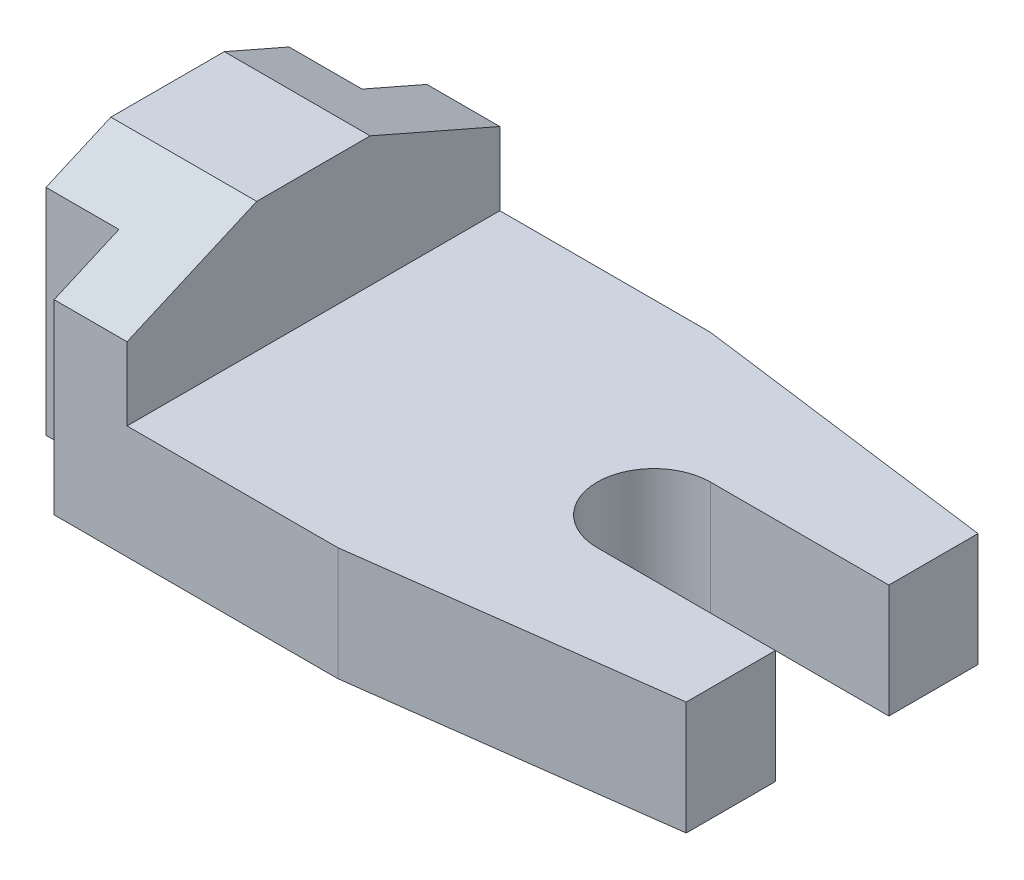
ISO-10303-21;
HEADER;
FILE_DESCRIPTION(('STEP AP214'),'2;1');
FILE_NAME('part.step','',(''),(''),'','','');
FILE_SCHEMA(('AUTOMOTIVE_DESIGN { 1 0 10303 214 1 1 1 1 }'));
ENDSEC;
DATA;
#1=APPLICATION_CONTEXT('core data for automotive mechanical design processes');
#2=APPLICATION_PROTOCOL_DEFINITION('international standard','automotive_design',2000,#1);
#3=PRODUCT_CONTEXT('',#1,'mechanical');
#4=PRODUCT('Part','Part','',(#3));
#5=PRODUCT_RELATED_PRODUCT_CATEGORY('part','',(#4));
#6=PRODUCT_DEFINITION_FORMATION('','',#4);
#7=PRODUCT_DEFINITION_CONTEXT('part definition',#1,'design');
#8=PRODUCT_DEFINITION('design','',#6,#7);
#9=PRODUCT_DEFINITION_SHAPE('','',#8);
#10=(LENGTH_UNIT() NAMED_UNIT(*) SI_UNIT(.MILLI.,.METRE.));
#11=(NAMED_UNIT(*) PLANE_ANGLE_UNIT() SI_UNIT($,.RADIAN.));
#12=(NAMED_UNIT(*) SI_UNIT($,.STERADIAN.) SOLID_ANGLE_UNIT());
#13=UNCERTAINTY_MEASURE_WITH_UNIT(LENGTH_MEASURE(1.E-05),#10,'distance_accuracy_value','');
#14=(GEOMETRIC_REPRESENTATION_CONTEXT(3) GLOBAL_UNCERTAINTY_ASSIGNED_CONTEXT((#13)) GLOBAL_UNIT_ASSIGNED_CONTEXT((#10,
#11,#12)) REPRESENTATION_CONTEXT('',''));
#15=CARTESIAN_POINT('',(0.,0.,0.));
#16=DIRECTION('',(0.,0.,1.));
#17=DIRECTION('',(1.,0.,0.));
#18=AXIS2_PLACEMENT_3D('',#15,#16,#17);
#19=CARTESIAN_POINT('',(0.,14.,0.));
#20=DIRECTION('',(0.,1.,0.));
#21=DIRECTION('',(0.,0.,1.));
#22=AXIS2_PLACEMENT_3D('',#19,#20,#21);
#23=PLANE('',#22);
#24=DIRECTION('',(1.,0.,0.));
#25=VECTOR('',#24,1.);
#26=CARTESIAN_POINT('',(0.,14.,-23.));
#27=LINE('',#26,#25);
#28=CARTESIAN_POINT('',(-4.,14.,-23.));
#29=VERTEX_POINT('',#28);
#30=CARTESIAN_POINT('',(22.,14.,-23.));
#31=VERTEX_POINT('',#30);
#32=EDGE_CURVE('E63',#29,#31,#27,.T.);
#33=ORIENTED_EDGE('',*,*,#32,.F.);
#34=DIRECTION('',(0.,0.,1.));
#35=VECTOR('',#34,1.);
#36=CARTESIAN_POINT('',(-4.,14.,0.));
#37=LINE('',#36,#35);
#38=CARTESIAN_POINT('',(-4.,14.,23.));
#39=VERTEX_POINT('',#38);
#40=EDGE_CURVE('E276',#29,#39,#37,.T.);
#41=ORIENTED_EDGE('',*,*,#40,.T.);
#42=DIRECTION('',(1.,0.,0.));
#43=VECTOR('',#42,1.);
#44=CARTESIAN_POINT('',(0.,14.,23.));
#45=LINE('',#44,#43);
#46=CARTESIAN_POINT('',(22.,14.,23.));
#47=VERTEX_POINT('',#46);
#48=EDGE_CURVE('E128',#39,#47,#45,.T.);
#49=ORIENTED_EDGE('',*,*,#48,.T.);
#50=DIRECTION('',(-0.991454295542544,0.,0.130454512571387));
#51=VECTOR('',#50,1.);
#52=CARTESIAN_POINT('',(3.34921715452689,14.,25.4540503744043));
#53=LINE('',#52,#51);
#54=CARTESIAN_POINT('',(60.,14.,18.));
#55=VERTEX_POINT('',#54);
#56=EDGE_CURVE('E253',#55,#47,#53,.T.);
#57=ORIENTED_EDGE('',*,*,#56,.F.);
#58=DIRECTION('',(0.,0.,1.));
#59=VECTOR('',#58,1.);
#60=CARTESIAN_POINT('',(60.,14.,0.));
#61=LINE('',#60,#59);
#62=CARTESIAN_POINT('',(60.,14.,7.));
#63=VERTEX_POINT('',#62);
#64=EDGE_CURVE('E257',#63,#55,#61,.T.);
#65=ORIENTED_EDGE('',*,*,#64,.F.);
#66=DIRECTION('',(-1.,0.,0.));
#67=VECTOR('',#66,1.);
#68=CARTESIAN_POINT('',(0.,14.,7.));
#69=LINE('',#68,#67);
#70=CARTESIAN_POINT('',(38.,14.,7.));
#71=VERTEX_POINT('',#70);
#72=EDGE_CURVE('E268',#63,#71,#69,.T.);
#73=ORIENTED_EDGE('',*,*,#72,.T.);
#74=CARTESIAN_POINT('',(38.,14.,0.));
#75=DIRECTION('',(0.,1.,0.));
#76=DIRECTION('',(0.,0.,1.));
#77=AXIS2_PLACEMENT_3D('',#74,#75,#76);
#78=CIRCLE('',#77,7.);
#79=CARTESIAN_POINT('',(38.,14.,-7.));
#80=VERTEX_POINT('',#79);
#81=EDGE_CURVE('E152',#80,#71,#78,.T.);
#82=ORIENTED_EDGE('',*,*,#81,.F.);
#83=DIRECTION('',(1.,0.,0.));
#84=VECTOR('',#83,1.);
#85=CARTESIAN_POINT('',(0.,14.,-7.));
#86=LINE('',#85,#84);
#87=CARTESIAN_POINT('',(60.,14.,-7.));
#88=VERTEX_POINT('',#87);
#89=EDGE_CURVE('E149',#80,#88,#86,.T.);
#90=ORIENTED_EDGE('',*,*,#89,.T.);
#91=DIRECTION('',(0.,0.,1.));
#92=VECTOR('',#91,1.);
#93=CARTESIAN_POINT('',(60.,14.,0.));
#94=LINE('',#93,#92);
#95=CARTESIAN_POINT('',(60.,14.,-18.));
#96=VERTEX_POINT('',#95);
#97=EDGE_CURVE('E155',#96,#88,#94,.T.);
#98=ORIENTED_EDGE('',*,*,#97,.F.);
#99=DIRECTION('',(-0.991454295542544,0.,-0.130454512571387));
#100=VECTOR('',#99,1.);
#101=CARTESIAN_POINT('',(3.34921715452689,14.,-25.4540503744044));
#102=LINE('',#101,#100);
#103=EDGE_CURVE('E168',#96,#31,#102,.T.);
#104=ORIENTED_EDGE('',*,*,#103,.T.);
#105=EDGE_LOOP('',(#33,#41,#49,#57,#65,#73,#82,#90,#98,#104));
#106=FACE_BOUND('',#105,.T.);
#107=ADVANCED_FACE('F50',(#106),#23,.T.);
#108=CARTESIAN_POINT('',(0.,14.,15.));
#109=DIRECTION('',(0.,0.,-1.));
#110=DIRECTION('',(-1.,0.,0.));
#111=AXIS2_PLACEMENT_3D('',#108,#109,#110);
#112=PLANE('',#111);
#113=DIRECTION('',(1.,0.,0.));
#114=VECTOR('',#113,1.);
#115=CARTESIAN_POINT('',(0.,0.,15.));
#116=LINE('',#115,#114);
#117=CARTESIAN_POINT('',(-22.,0.,15.));
#118=VERTEX_POINT('',#117);
#119=CARTESIAN_POINT('',(-13.,0.,15.));
#120=VERTEX_POINT('',#119);
#121=EDGE_CURVE('E176',#118,#120,#116,.T.);
#122=ORIENTED_EDGE('',*,*,#121,.T.);
#123=DIRECTION('',(0.,-1.,0.));
#124=VECTOR('',#123,1.);
#125=CARTESIAN_POINT('',(-13.,14.,15.));
#126=LINE('',#125,#124);
#127=CARTESIAN_POINT('',(-13.,26.5,15.));
#128=VERTEX_POINT('',#127);
#129=EDGE_CURVE('E11',#128,#120,#126,.T.);
#130=ORIENTED_EDGE('',*,*,#129,.F.);
#131=DIRECTION('',(-1.,0.,0.));
#132=VECTOR('',#131,1.);
#133=CARTESIAN_POINT('',(-13.,26.5,15.));
#134=LINE('',#133,#132);
#135=CARTESIAN_POINT('',(-22.,26.5,15.));
#136=VERTEX_POINT('',#135);
#137=EDGE_CURVE('E177',#128,#136,#134,.T.);
#138=ORIENTED_EDGE('',*,*,#137,.T.);
#139=DIRECTION('',(0.,-1.,0.));
#140=VECTOR('',#139,1.);
#141=CARTESIAN_POINT('',(-22.,14.,15.));
#142=LINE('',#141,#140);
#143=EDGE_CURVE('E121',#136,#118,#142,.T.);
#144=ORIENTED_EDGE('',*,*,#143,.T.);
#145=EDGE_LOOP('',(#122,#130,#138,#144));
#146=FACE_BOUND('',#145,.T.);
#147=ADVANCED_FACE('F47',(#146),#112,.F.);
#148=CARTESIAN_POINT('',(-13.,14.,0.));
#149=DIRECTION('',(1.,0.,0.));
#150=DIRECTION('',(0.,0.,-1.));
#151=AXIS2_PLACEMENT_3D('',#148,#149,#150);
#152=PLANE('',#151);
#153=DIRECTION('',(0.,0.,1.));
#154=VECTOR('',#153,1.);
#155=CARTESIAN_POINT('',(-13.,0.,0.));
#156=LINE('',#155,#154);
#157=CARTESIAN_POINT('',(-13.,0.,23.));
#158=VERTEX_POINT('',#157);
#159=EDGE_CURVE('E178',#120,#158,#156,.T.);
#160=ORIENTED_EDGE('',*,*,#159,.T.);
#161=DIRECTION('',(0.,-1.,0.));
#162=VECTOR('',#161,1.);
#163=CARTESIAN_POINT('',(-13.,14.,23.));
#164=LINE('',#163,#162);
#165=CARTESIAN_POINT('',(-13.,23.,23.));
#166=VERTEX_POINT('',#165);
#167=EDGE_CURVE('E57',#166,#158,#164,.T.);
#168=ORIENTED_EDGE('',*,*,#167,.F.);
#169=DIRECTION('',(0.,0.400818834019708,-0.916157334902189));
#170=VECTOR('',#169,1.);
#171=CARTESIAN_POINT('',(-13.,30.,7.));
#172=LINE('',#171,#170);
#173=EDGE_CURVE('E356',#166,#128,#172,.T.);
#174=ORIENTED_EDGE('',*,*,#173,.T.);
#175=ORIENTED_EDGE('',*,*,#129,.T.);
#176=EDGE_LOOP('',(#160,#168,#174,#175));
#177=FACE_BOUND('',#176,.T.);
#178=ADVANCED_FACE('F379',(#177),#152,.F.);
#179=CARTESIAN_POINT('',(0.,14.,23.));
#180=DIRECTION('',(0.,0.,-1.));
#181=DIRECTION('',(-1.,0.,0.));
#182=AXIS2_PLACEMENT_3D('',#179,#180,#181);
#183=PLANE('',#182);
#184=DIRECTION('',(1.,0.,0.));
#185=VECTOR('',#184,1.);
#186=CARTESIAN_POINT('',(0.,0.,23.));
#187=LINE('',#186,#185);
#188=CARTESIAN_POINT('',(22.,0.,23.));
#189=VERTEX_POINT('',#188);
#190=EDGE_CURVE('E182',#158,#189,#187,.T.);
#191=ORIENTED_EDGE('',*,*,#190,.T.);
#192=DIRECTION('',(0.,-1.,0.));
#193=VECTOR('',#192,1.);
#194=CARTESIAN_POINT('',(22.,14.,23.));
#195=LINE('',#194,#193);
#196=EDGE_CURVE('E230',#47,#189,#195,.T.);
#197=ORIENTED_EDGE('',*,*,#196,.F.);
#198=ORIENTED_EDGE('',*,*,#48,.F.);
#199=DIRECTION('',(0.,1.,0.));
#200=VECTOR('',#199,1.);
#201=CARTESIAN_POINT('',(-4.,0.,23.));
#202=LINE('',#201,#200);
#203=CARTESIAN_POINT('',(-4.,23.,23.));
#204=VERTEX_POINT('',#203);
#205=EDGE_CURVE('E254',#39,#204,#202,.T.);
#206=ORIENTED_EDGE('',*,*,#205,.T.);
#207=DIRECTION('',(-1.,0.,0.));
#208=VECTOR('',#207,1.);
#209=CARTESIAN_POINT('',(-4.,23.,23.));
#210=LINE('',#209,#208);
#211=EDGE_CURVE('E239',#204,#166,#210,.T.);
#212=ORIENTED_EDGE('',*,*,#211,.T.);
#213=ORIENTED_EDGE('',*,*,#167,.T.);
#214=EDGE_LOOP('',(#191,#197,#198,#206,#212,#213));
#215=FACE_BOUND('',#214,.T.);
#216=ADVANCED_FACE('F234',(#215),#183,.F.);
#217=CARTESIAN_POINT('',(3.34921715452689,14.,25.4540503744043));
#218=DIRECTION('',(0.130454512571387,0.,0.991454295542544));
#219=DIRECTION('',(0.991454295542544,0.,-0.130454512571387));
#220=AXIS2_PLACEMENT_3D('',#217,#218,#219);
#221=PLANE('',#220);
#222=DIRECTION('',(-0.991454295542544,0.,0.130454512571387));
#223=VECTOR('',#222,1.);
#224=CARTESIAN_POINT('',(3.34921715452689,0.,25.4540503744043));
#225=LINE('',#224,#223);
#226=CARTESIAN_POINT('',(60.,0.,18.));
#227=VERTEX_POINT('',#226);
#228=EDGE_CURVE('E181',#227,#189,#225,.T.);
#229=ORIENTED_EDGE('',*,*,#228,.F.);
#230=DIRECTION('',(0.,-1.,0.));
#231=VECTOR('',#230,1.);
#232=CARTESIAN_POINT('',(60.,14.,18.));
#233=LINE('',#232,#231);
#234=EDGE_CURVE('E229',#55,#227,#233,.T.);
#235=ORIENTED_EDGE('',*,*,#234,.F.);
#236=ORIENTED_EDGE('',*,*,#56,.T.);
#237=ORIENTED_EDGE('',*,*,#196,.T.);
#238=EDGE_LOOP('',(#229,#235,#236,#237));
#239=FACE_BOUND('',#238,.T.);
#240=ADVANCED_FACE('F247',(#239),#221,.T.);
#241=CARTESIAN_POINT('',(60.,14.,0.));
#242=DIRECTION('',(1.,0.,0.));
#243=DIRECTION('',(0.,0.,-1.));
#244=AXIS2_PLACEMENT_3D('',#241,#242,#243);
#245=PLANE('',#244);
#246=DIRECTION('',(0.,0.,1.));
#247=VECTOR('',#246,1.);
#248=CARTESIAN_POINT('',(60.,0.,0.));
#249=LINE('',#248,#247);
#250=CARTESIAN_POINT('',(60.,0.,7.));
#251=VERTEX_POINT('',#250);
#252=EDGE_CURVE('E189',#251,#227,#249,.T.);
#253=ORIENTED_EDGE('',*,*,#252,.F.);
#254=DIRECTION('',(0.,-1.,0.));
#255=VECTOR('',#254,1.);
#256=CARTESIAN_POINT('',(60.,14.,7.));
#257=LINE('',#256,#255);
#258=EDGE_CURVE('E221',#63,#251,#257,.T.);
#259=ORIENTED_EDGE('',*,*,#258,.F.);
#260=ORIENTED_EDGE('',*,*,#64,.T.);
#261=ORIENTED_EDGE('',*,*,#234,.T.);
#262=EDGE_LOOP('',(#253,#259,#260,#261));
#263=FACE_BOUND('',#262,.T.);
#264=ADVANCED_FACE('F437',(#263),#245,.T.);
#265=CARTESIAN_POINT('',(0.,14.,7.));
#266=DIRECTION('',(0.,0.,1.));
#267=DIRECTION('',(1.,0.,0.));
#268=AXIS2_PLACEMENT_3D('',#265,#266,#267);
#269=PLANE('',#268);
#270=DIRECTION('',(-1.,0.,0.));
#271=VECTOR('',#270,1.);
#272=CARTESIAN_POINT('',(0.,0.,7.));
#273=LINE('',#272,#271);
#274=CARTESIAN_POINT('',(38.,0.,7.));
#275=VERTEX_POINT('',#274);
#276=EDGE_CURVE('E188',#251,#275,#273,.T.);
#277=ORIENTED_EDGE('',*,*,#276,.T.);
#278=DIRECTION('',(0.,-1.,0.));
#279=VECTOR('',#278,1.);
#280=CARTESIAN_POINT('',(38.,14.,7.));
#281=LINE('',#280,#279);
#282=EDGE_CURVE('E225',#71,#275,#281,.T.);
#283=ORIENTED_EDGE('',*,*,#282,.F.);
#284=ORIENTED_EDGE('',*,*,#72,.F.);
#285=ORIENTED_EDGE('',*,*,#258,.T.);
#286=EDGE_LOOP('',(#277,#283,#284,#285));
#287=FACE_BOUND('',#286,.T.);
#288=ADVANCED_FACE('F426',(#287),#269,.F.);
#289=CARTESIAN_POINT('',(38.,14.,0.));
#290=DIRECTION('',(0.,-1.,0.));
#291=DIRECTION('',(0.,0.,-1.));
#292=AXIS2_PLACEMENT_3D('',#289,#290,#291);
#293=CYLINDRICAL_SURFACE('',#292,7.);
#294=CARTESIAN_POINT('',(38.,0.,0.));
#295=DIRECTION('',(0.,1.,0.));
#296=DIRECTION('',(0.,0.,1.));
#297=AXIS2_PLACEMENT_3D('',#294,#295,#296);
#298=CIRCLE('',#297,7.);
#299=CARTESIAN_POINT('',(38.,0.,-7.));
#300=VERTEX_POINT('',#299);
#301=EDGE_CURVE('E195',#300,#275,#298,.T.);
#302=ORIENTED_EDGE('',*,*,#301,.F.);
#303=DIRECTION('',(0.,-1.,0.));
#304=VECTOR('',#303,1.);
#305=CARTESIAN_POINT('',(38.,14.,-7.));
#306=LINE('',#305,#304);
#307=EDGE_CURVE('E164',#80,#300,#306,.T.);
#308=ORIENTED_EDGE('',*,*,#307,.F.);
#309=ORIENTED_EDGE('',*,*,#81,.T.);
#310=ORIENTED_EDGE('',*,*,#282,.T.);
#311=EDGE_LOOP('',(#302,#308,#309,#310));
#312=FACE_BOUND('',#311,.T.);
#313=ADVANCED_FACE('F271',(#312),#293,.F.);
#314=CARTESIAN_POINT('',(0.,14.,-7.));
#315=DIRECTION('',(0.,0.,-1.));
#316=DIRECTION('',(-1.,0.,0.));
#317=AXIS2_PLACEMENT_3D('',#314,#315,#316);
#318=PLANE('',#317);
#319=DIRECTION('',(1.,0.,0.));
#320=VECTOR('',#319,1.);
#321=CARTESIAN_POINT('',(0.,0.,-7.));
#322=LINE('',#321,#320);
#323=CARTESIAN_POINT('',(60.,0.,-7.));
#324=VERTEX_POINT('',#323);
#325=EDGE_CURVE('E161',#300,#324,#322,.T.);
#326=ORIENTED_EDGE('',*,*,#325,.T.);
#327=DIRECTION('',(0.,-1.,0.));
#328=VECTOR('',#327,1.);
#329=CARTESIAN_POINT('',(60.,14.,-7.));
#330=LINE('',#329,#328);
#331=EDGE_CURVE('E158',#88,#324,#330,.T.);
#332=ORIENTED_EDGE('',*,*,#331,.F.);
#333=ORIENTED_EDGE('',*,*,#89,.F.);
#334=ORIENTED_EDGE('',*,*,#307,.T.);
#335=EDGE_LOOP('',(#326,#332,#333,#334));
#336=FACE_BOUND('',#335,.T.);
#337=ADVANCED_FACE('F157',(#336),#318,.F.);
#338=CARTESIAN_POINT('',(60.,14.,0.));
#339=DIRECTION('',(1.,0.,0.));
#340=DIRECTION('',(0.,0.,-1.));
#341=AXIS2_PLACEMENT_3D('',#338,#339,#340);
#342=PLANE('',#341);
#343=DIRECTION('',(0.,0.,1.));
#344=VECTOR('',#343,1.);
#345=CARTESIAN_POINT('',(60.,0.,0.));
#346=LINE('',#345,#344);
#347=CARTESIAN_POINT('',(60.,0.,-18.));
#348=VERTEX_POINT('',#347);
#349=EDGE_CURVE('E198',#348,#324,#346,.T.);
#350=ORIENTED_EDGE('',*,*,#349,.F.);
#351=DIRECTION('',(0.,-1.,0.));
#352=VECTOR('',#351,1.);
#353=CARTESIAN_POINT('',(60.,14.,-18.));
#354=LINE('',#353,#352);
#355=EDGE_CURVE('E167',#96,#348,#354,.T.);
#356=ORIENTED_EDGE('',*,*,#355,.F.);
#357=ORIENTED_EDGE('',*,*,#97,.T.);
#358=ORIENTED_EDGE('',*,*,#331,.T.);
#359=EDGE_LOOP('',(#350,#356,#357,#358));
#360=FACE_BOUND('',#359,.T.);
#361=ADVANCED_FACE('F169',(#360),#342,.T.);
#362=CARTESIAN_POINT('',(3.34921715452689,14.,-25.4540503744044));
#363=DIRECTION('',(-0.130454512571387,0.,0.991454295542544));
#364=DIRECTION('',(0.991454295542544,0.,0.130454512571387));
#365=AXIS2_PLACEMENT_3D('',#362,#363,#364);
#366=PLANE('',#365);
#367=DIRECTION('',(-0.991454295542544,0.,-0.130454512571387));
#368=VECTOR('',#367,1.);
#369=CARTESIAN_POINT('',(3.34921715452689,0.,-25.4540503744044));
#370=LINE('',#369,#368);
#371=CARTESIAN_POINT('',(22.,0.,-23.));
#372=VERTEX_POINT('',#371);
#373=EDGE_CURVE('E196',#348,#372,#370,.T.);
#374=ORIENTED_EDGE('',*,*,#373,.T.);
#375=DIRECTION('',(0.,-1.,0.));
#376=VECTOR('',#375,1.);
#377=CARTESIAN_POINT('',(22.,14.,-23.));
#378=LINE('',#377,#376);
#379=EDGE_CURVE('E217',#31,#372,#378,.T.);
#380=ORIENTED_EDGE('',*,*,#379,.F.);
#381=ORIENTED_EDGE('',*,*,#103,.F.);
#382=ORIENTED_EDGE('',*,*,#355,.T.);
#383=EDGE_LOOP('',(#374,#380,#381,#382));
#384=FACE_BOUND('',#383,.T.);
#385=ADVANCED_FACE('F280',(#384),#366,.F.);
#386=CARTESIAN_POINT('',(0.,14.,-23.));
#387=DIRECTION('',(0.,0.,-1.));
#388=DIRECTION('',(-1.,0.,0.));
#389=AXIS2_PLACEMENT_3D('',#386,#387,#388);
#390=PLANE('',#389);
#391=DIRECTION('',(0.,-1.,0.));
#392=VECTOR('',#391,1.);
#393=CARTESIAN_POINT('',(-13.,14.,-23.));
#394=LINE('',#393,#392);
#395=CARTESIAN_POINT('',(-13.,23.,-23.));
#396=VERTEX_POINT('',#395);
#397=CARTESIAN_POINT('',(-13.,0.,-23.));
#398=VERTEX_POINT('',#397);
#399=EDGE_CURVE('E216',#396,#398,#394,.T.);
#400=ORIENTED_EDGE('',*,*,#399,.F.);
#401=DIRECTION('',(-1.,0.,0.));
#402=VECTOR('',#401,1.);
#403=CARTESIAN_POINT('',(-4.,23.,-23.));
#404=LINE('',#403,#402);
#405=CARTESIAN_POINT('',(-4.,23.,-23.));
#406=VERTEX_POINT('',#405);
#407=EDGE_CURVE('E348',#406,#396,#404,.T.);
#408=ORIENTED_EDGE('',*,*,#407,.F.);
#409=DIRECTION('',(0.,-1.,0.));
#410=VECTOR('',#409,1.);
#411=CARTESIAN_POINT('',(-4.,23.,-23.));
#412=LINE('',#411,#410);
#413=EDGE_CURVE('E351',#406,#29,#412,.T.);
#414=ORIENTED_EDGE('',*,*,#413,.T.);
#415=ORIENTED_EDGE('',*,*,#32,.T.);
#416=ORIENTED_EDGE('',*,*,#379,.T.);
#417=DIRECTION('',(1.,0.,0.));
#418=VECTOR('',#417,1.);
#419=CARTESIAN_POINT('',(0.,0.,-23.));
#420=LINE('',#419,#418);
#421=EDGE_CURVE('E203',#398,#372,#420,.T.);
#422=ORIENTED_EDGE('',*,*,#421,.F.);
#423=EDGE_LOOP('',(#400,#408,#414,#415,#416,#422));
#424=FACE_BOUND('',#423,.T.);
#425=ADVANCED_FACE('F354',(#424),#390,.T.);
#426=CARTESIAN_POINT('',(-13.,14.,0.));
#427=DIRECTION('',(-1.,0.,0.));
#428=DIRECTION('',(0.,0.,1.));
#429=AXIS2_PLACEMENT_3D('',#426,#427,#428);
#430=PLANE('',#429);
#431=DIRECTION('',(0.,0.,-1.));
#432=VECTOR('',#431,1.);
#433=CARTESIAN_POINT('',(-13.,0.,0.));
#434=LINE('',#433,#432);
#435=CARTESIAN_POINT('',(-13.,0.,-15.));
#436=VERTEX_POINT('',#435);
#437=EDGE_CURVE('E201',#436,#398,#434,.T.);
#438=ORIENTED_EDGE('',*,*,#437,.F.);
#439=DIRECTION('',(0.,-1.,0.));
#440=VECTOR('',#439,1.);
#441=CARTESIAN_POINT('',(-13.,14.,-15.));
#442=LINE('',#441,#440);
#443=CARTESIAN_POINT('',(-13.,26.5,-15.));
#444=VERTEX_POINT('',#443);
#445=EDGE_CURVE('E212',#444,#436,#442,.T.);
#446=ORIENTED_EDGE('',*,*,#445,.F.);
#447=DIRECTION('',(0.,-0.400818834019708,-0.916157334902189));
#448=VECTOR('',#447,1.);
#449=CARTESIAN_POINT('',(-13.,23.,-23.));
#450=LINE('',#449,#448);
#451=EDGE_CURVE('E334',#444,#396,#450,.T.);
#452=ORIENTED_EDGE('',*,*,#451,.T.);
#453=ORIENTED_EDGE('',*,*,#399,.T.);
#454=EDGE_LOOP('',(#438,#446,#452,#453));
#455=FACE_BOUND('',#454,.T.);
#456=ADVANCED_FACE('F364',(#455),#430,.T.);
#457=CARTESIAN_POINT('',(0.,14.,-15.));
#458=DIRECTION('',(0.,0.,-1.));
#459=DIRECTION('',(-1.,0.,0.));
#460=AXIS2_PLACEMENT_3D('',#457,#458,#459);
#461=PLANE('',#460);
#462=DIRECTION('',(1.,0.,0.));
#463=VECTOR('',#462,1.);
#464=CARTESIAN_POINT('',(0.,0.,-15.));
#465=LINE('',#464,#463);
#466=CARTESIAN_POINT('',(-22.,0.,-15.));
#467=VERTEX_POINT('',#466);
#468=EDGE_CURVE('E206',#467,#436,#465,.T.);
#469=ORIENTED_EDGE('',*,*,#468,.F.);
#470=DIRECTION('',(0.,-1.,0.));
#471=VECTOR('',#470,1.);
#472=CARTESIAN_POINT('',(-22.,14.,-15.));
#473=LINE('',#472,#471);
#474=CARTESIAN_POINT('',(-22.,26.5,-15.));
#475=VERTEX_POINT('',#474);
#476=EDGE_CURVE('E114',#475,#467,#473,.T.);
#477=ORIENTED_EDGE('',*,*,#476,.F.);
#478=DIRECTION('',(-1.,0.,0.));
#479=VECTOR('',#478,1.);
#480=CARTESIAN_POINT('',(-13.,26.5,-15.));
#481=LINE('',#480,#479);
#482=EDGE_CURVE('E303',#444,#475,#481,.T.);
#483=ORIENTED_EDGE('',*,*,#482,.F.);
#484=ORIENTED_EDGE('',*,*,#445,.T.);
#485=EDGE_LOOP('',(#469,#477,#483,#484));
#486=FACE_BOUND('',#485,.T.);
#487=ADVANCED_FACE('F331',(#486),#461,.T.);
#488=CARTESIAN_POINT('',(-22.,14.,0.));
#489=DIRECTION('',(-1.,0.,0.));
#490=DIRECTION('',(0.,0.,1.));
#491=AXIS2_PLACEMENT_3D('',#488,#489,#490);
#492=PLANE('',#491);
#493=DIRECTION('',(0.,0.,-1.));
#494=VECTOR('',#493,1.);
#495=CARTESIAN_POINT('',(-22.,0.,0.));
#496=LINE('',#495,#494);
#497=EDGE_CURVE('E207',#118,#467,#496,.T.);
#498=ORIENTED_EDGE('',*,*,#497,.F.);
#499=ORIENTED_EDGE('',*,*,#143,.F.);
#500=DIRECTION('',(0.,0.400818834019708,-0.916157334902189));
#501=VECTOR('',#500,1.);
#502=CARTESIAN_POINT('',(-22.,30.,7.));
#503=LINE('',#502,#501);
#504=CARTESIAN_POINT('',(-22.,30.,7.));
#505=VERTEX_POINT('',#504);
#506=EDGE_CURVE('E300',#136,#505,#503,.T.);
#507=ORIENTED_EDGE('',*,*,#506,.T.);
#508=DIRECTION('',(0.,0.,-1.));
#509=VECTOR('',#508,1.);
#510=CARTESIAN_POINT('',(-22.,30.,7.));
#511=LINE('',#510,#509);
#512=CARTESIAN_POINT('',(-22.,30.,-7.));
#513=VERTEX_POINT('',#512);
#514=EDGE_CURVE('E310',#505,#513,#511,.T.);
#515=ORIENTED_EDGE('',*,*,#514,.T.);
#516=DIRECTION('',(0.,-0.400818834019708,-0.916157334902189));
#517=VECTOR('',#516,1.);
#518=CARTESIAN_POINT('',(-22.,26.5,-15.));
#519=LINE('',#518,#517);
#520=EDGE_CURVE('E313',#513,#475,#519,.T.);
#521=ORIENTED_EDGE('',*,*,#520,.T.);
#522=ORIENTED_EDGE('',*,*,#476,.T.);
#523=EDGE_LOOP('',(#498,#499,#507,#515,#521,#522));
#524=FACE_BOUND('',#523,.T.);
#525=ADVANCED_FACE('F293',(#524),#492,.T.);
#526=CARTESIAN_POINT('',(0.,0.,0.));
#527=DIRECTION('',(0.,1.,0.));
#528=DIRECTION('',(0.,0.,1.));
#529=AXIS2_PLACEMENT_3D('',#526,#527,#528);
#530=PLANE('',#529);
#531=ORIENTED_EDGE('',*,*,#468,.T.);
#532=ORIENTED_EDGE('',*,*,#437,.T.);
#533=ORIENTED_EDGE('',*,*,#421,.T.);
#534=ORIENTED_EDGE('',*,*,#373,.F.);
#535=ORIENTED_EDGE('',*,*,#349,.T.);
#536=ORIENTED_EDGE('',*,*,#325,.F.);
#537=ORIENTED_EDGE('',*,*,#301,.T.);
#538=ORIENTED_EDGE('',*,*,#276,.F.);
#539=ORIENTED_EDGE('',*,*,#252,.T.);
#540=ORIENTED_EDGE('',*,*,#228,.T.);
#541=ORIENTED_EDGE('',*,*,#190,.F.);
#542=ORIENTED_EDGE('',*,*,#159,.F.);
#543=ORIENTED_EDGE('',*,*,#121,.F.);
#544=ORIENTED_EDGE('',*,*,#497,.T.);
#545=EDGE_LOOP('',(#531,#532,#533,#534,#535,#536,#537,#538,#539,#540,#541,#542,#543,#544));
#546=FACE_BOUND('',#545,.T.);
#547=ADVANCED_FACE('F243',(#546),#530,.F.);
#548=CARTESIAN_POINT('',(-13.,30.,7.));
#549=DIRECTION('',(0.,0.916157334902189,0.400818834019708));
#550=DIRECTION('',(0.,-0.400818834019708,0.916157334902189));
#551=AXIS2_PLACEMENT_3D('',#548,#549,#550);
#552=PLANE('',#551);
#553=ORIENTED_EDGE('',*,*,#506,.F.);
#554=ORIENTED_EDGE('',*,*,#137,.F.);
#555=ORIENTED_EDGE('',*,*,#173,.F.);
#556=ORIENTED_EDGE('',*,*,#211,.F.);
#557=DIRECTION('',(0.,0.400818834019708,-0.916157334902189));
#558=VECTOR('',#557,1.);
#559=CARTESIAN_POINT('',(-4.,30.,7.));
#560=LINE('',#559,#558);
#561=CARTESIAN_POINT('',(-4.,30.,7.));
#562=VERTEX_POINT('',#561);
#563=EDGE_CURVE('E363',#204,#562,#560,.T.);
#564=ORIENTED_EDGE('',*,*,#563,.T.);
#565=DIRECTION('',(-1.,0.,0.));
#566=VECTOR('',#565,1.);
#567=CARTESIAN_POINT('',(-13.,30.,7.));
#568=LINE('',#567,#566);
#569=EDGE_CURVE('E263',#562,#505,#568,.T.);
#570=ORIENTED_EDGE('',*,*,#569,.T.);
#571=EDGE_LOOP('',(#553,#554,#555,#556,#564,#570));
#572=FACE_BOUND('',#571,.T.);
#573=ADVANCED_FACE('F304',(#572),#552,.T.);
#574=CARTESIAN_POINT('',(-13.,26.5,-15.));
#575=DIRECTION('',(0.,0.916157334902189,-0.400818834019708));
#576=DIRECTION('',(0.,0.400818834019708,0.916157334902189));
#577=AXIS2_PLACEMENT_3D('',#574,#575,#576);
#578=PLANE('',#577);
#579=ORIENTED_EDGE('',*,*,#520,.F.);
#580=DIRECTION('',(-1.,0.,0.));
#581=VECTOR('',#580,1.);
#582=CARTESIAN_POINT('',(-13.,30.,-7.));
#583=LINE('',#582,#581);
#584=CARTESIAN_POINT('',(-4.,30.,-7.));
#585=VERTEX_POINT('',#584);
#586=EDGE_CURVE('E320',#585,#513,#583,.T.);
#587=ORIENTED_EDGE('',*,*,#586,.F.);
#588=DIRECTION('',(0.,-0.400818834019708,-0.916157334902189));
#589=VECTOR('',#588,1.);
#590=CARTESIAN_POINT('',(-4.,23.,-23.));
#591=LINE('',#590,#589);
#592=EDGE_CURVE('E353',#585,#406,#591,.T.);
#593=ORIENTED_EDGE('',*,*,#592,.T.);
#594=ORIENTED_EDGE('',*,*,#407,.T.);
#595=ORIENTED_EDGE('',*,*,#451,.F.);
#596=ORIENTED_EDGE('',*,*,#482,.T.);
#597=EDGE_LOOP('',(#579,#587,#593,#594,#595,#596));
#598=FACE_BOUND('',#597,.T.);
#599=ADVANCED_FACE('F328',(#598),#578,.T.);
#600=CARTESIAN_POINT('',(-13.,30.,7.));
#601=DIRECTION('',(0.,1.,0.));
#602=DIRECTION('',(0.,0.,1.));
#603=AXIS2_PLACEMENT_3D('',#600,#601,#602);
#604=PLANE('',#603);
#605=ORIENTED_EDGE('',*,*,#514,.F.);
#606=ORIENTED_EDGE('',*,*,#569,.F.);
#607=DIRECTION('',(0.,0.,-1.));
#608=VECTOR('',#607,1.);
#609=CARTESIAN_POINT('',(-4.,30.,-7.));
#610=LINE('',#609,#608);
#611=EDGE_CURVE('E324',#562,#585,#610,.T.);
#612=ORIENTED_EDGE('',*,*,#611,.T.);
#613=ORIENTED_EDGE('',*,*,#586,.T.);
#614=EDGE_LOOP('',(#605,#606,#612,#613));
#615=FACE_BOUND('',#614,.T.);
#616=ADVANCED_FACE('F325',(#615),#604,.T.);
#617=CARTESIAN_POINT('',(-4.,0.,0.));
#618=DIRECTION('',(-1.,0.,0.));
#619=DIRECTION('',(0.,0.,1.));
#620=AXIS2_PLACEMENT_3D('',#617,#618,#619);
#621=PLANE('',#620);
#622=ORIENTED_EDGE('',*,*,#40,.F.);
#623=ORIENTED_EDGE('',*,*,#413,.F.);
#624=ORIENTED_EDGE('',*,*,#592,.F.);
#625=ORIENTED_EDGE('',*,*,#611,.F.);
#626=ORIENTED_EDGE('',*,*,#563,.F.);
#627=ORIENTED_EDGE('',*,*,#205,.F.);
#628=EDGE_LOOP('',(#622,#623,#624,#625,#626,#627));
#629=FACE_BOUND('',#628,.T.);
#630=ADVANCED_FACE('F355',(#629),#621,.F.);
#631=CLOSED_SHELL('',(#107,#147,#178,#216,#240,#264,#288,#313,#337,#361,#385,#425,#456,#487,
#525,#547,#573,#599,#616,#630));
#632=MANIFOLD_SOLID_BREP('B2',#631);
#633=ADVANCED_BREP_SHAPE_REPRESENTATION('',(#18,#632),#14);
#634=SHAPE_DEFINITION_REPRESENTATION(#9,#633);
ENDSEC;
END-ISO-10303-21;
